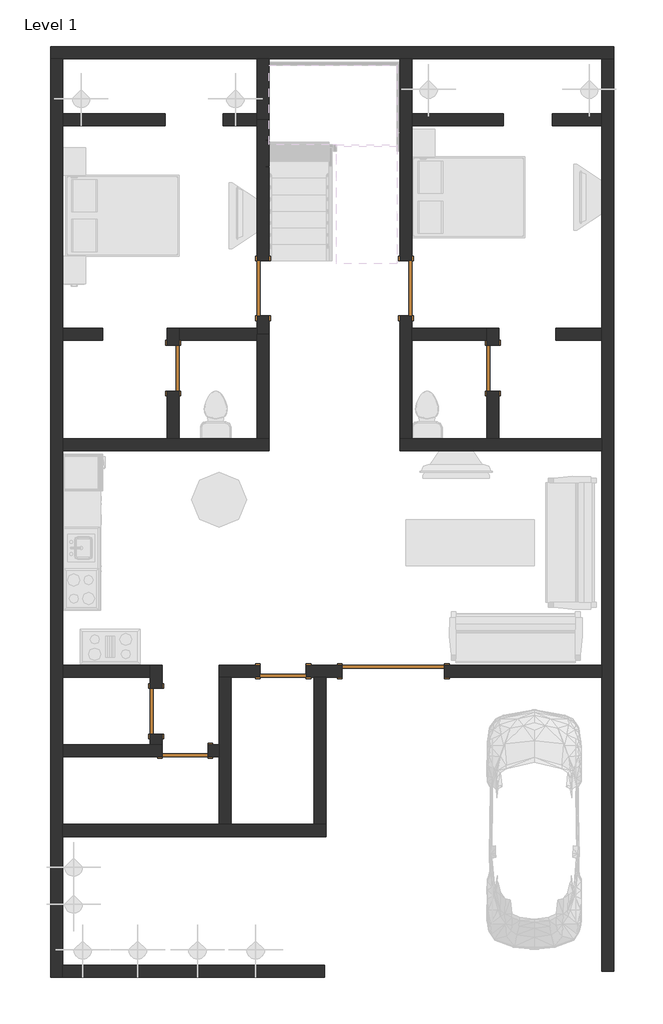
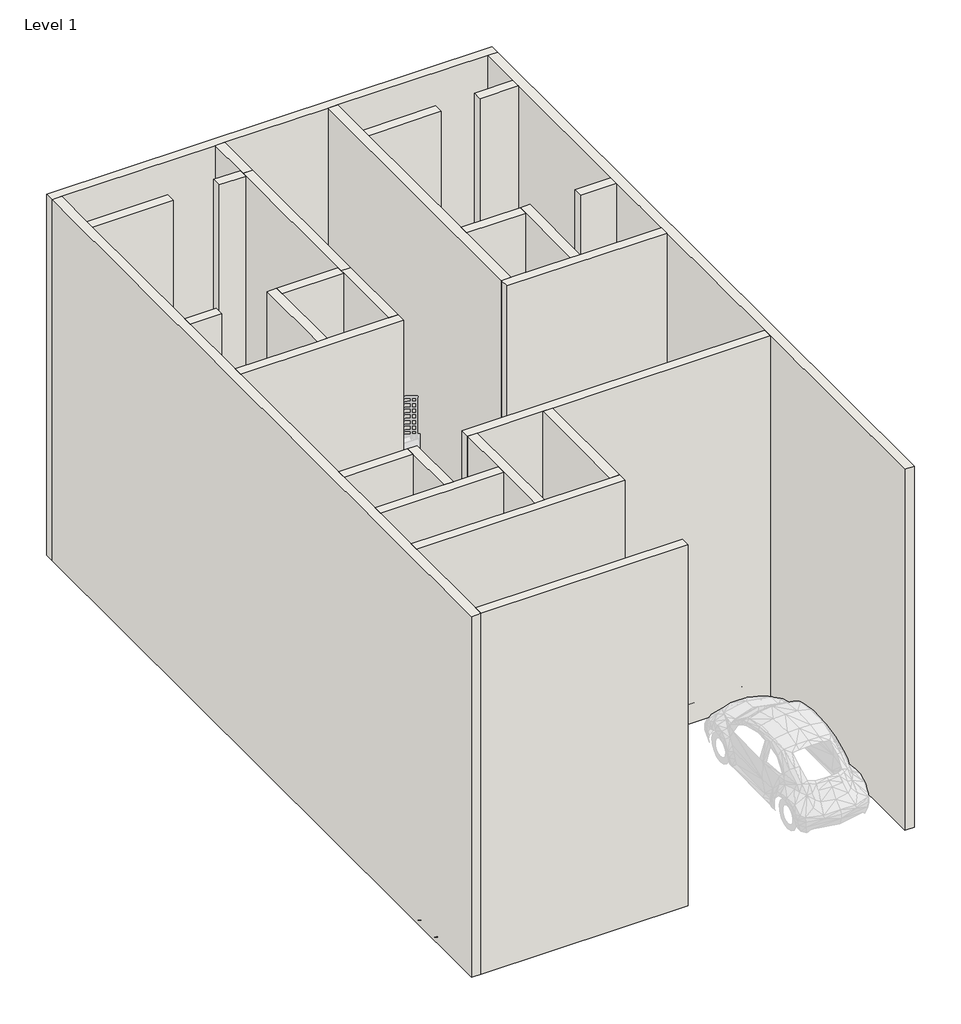
# One storey, part 1 of 4: 27 walls, 8 doors.
"""IFC4 building model written with IfcOpenShell, lengths in millimetres."""

from ifc_helpers import new_model, si_unit, origin, origin_with_axes, place, context, project, spatial, polyline, outline, extrude, faceted_brep, transform, mapped, element, save
from components import m_door_double_flush_panel_double_acting_1700_x_2000mm_0a6d9c7f, m_single_flush_0762_x_2032mm_7341a4fb, m_single_flush_0762_x_2032mm_0c256fab, m_single_flush_0915_x_2134mm_727434cd, m_single_flush_0915_x_2134mm_6a9e8738

model = new_model("IFC4")

# Units and contexts
model_context = context("Model", 3, world=origin())
ifc_project = project(units=[si_unit("LENGTHUNIT", "METRE", prefix="MILLI")], contexts=[model_context])

# Site, building, storey
site = spatial("IfcSite", under=ifc_project)
building = spatial("IfcBuilding", under=site)
storey = spatial("IfcBuildingStorey", under=building, Name="Level 1", Elevation=0.0)

# Doors
placement = place(None, origin())
m_door_double_flush_panel_double_acting_1700_x_2000mm_shape = m_door_double_flush_panel_double_acting_1700_x_2000mm_0a6d9c7f(model_context)
element("IfcDoor", 1, ObjectType="M_Door-Double-Flush_Panel-Double-Acting : 1700 x 2000mm", at=placement, inside=storey, context=model_context, shape_type="MappedRepresentation", body=[
    mapped(m_door_double_flush_panel_double_acting_1700_x_2000mm_shape, transform((-2495.9697318, 2089.9482221, 0.0), x_axis=(1.0, 0.0, 0.0), y_axis=(0.0, 1.0, 0.0), z_axis=(0.0, 0.0, 1.0))),
])
m_single_flush_0762_x_2032mm_shape = m_single_flush_0762_x_2032mm_7341a4fb(model_context)
element("IfcDoor", 2, ObjectType="M_Single-Flush : 0762 x 2032mm", at=placement, inside=storey, context=model_context, shape_type="MappedRepresentation", body=[
    mapped(m_single_flush_0762_x_2032mm_shape, transform((-6155.1697318, 7120.7482221, 0.0), x_axis=(0.0, 1.0, 0.0), y_axis=(-1.0, 0.0, 0.0), z_axis=(0.0, 0.0, 1.0))),
])
element("IfcDoor", 3, ObjectType="M_Single-Flush : 0762 x 2032mm", at=placement, inside=storey, context=model_context, shape_type="MappedRepresentation", body=[
    mapped(m_single_flush_0762_x_2032mm_shape, transform((-5951.9697318, 770.7482221, 0.0), x_axis=(1.0, 0.0, 0.0), y_axis=(0.0, 1.0, 0.0), z_axis=(0.0, 0.0, 1.0))),
])
element("IfcDoor", 4, ObjectType="M_Single-Flush : 0762 x 2032mm", at=placement, inside=storey, context=model_context, shape_type="MappedRepresentation", body=[
    mapped(m_single_flush_0762_x_2032mm_shape, transform((-4324.7697318, 2089.9482221, 0.0), x_axis=(1.0, 0.0, 0.0), y_axis=(0.0, 1.0, 0.0), z_axis=(0.0, 0.0, 1.0))),
])
m_single_flush_0762_x_2032mm_2_shape = m_single_flush_0762_x_2032mm_0c256fab(model_context)
element("IfcDoor", 5, ObjectType="M_Single-Flush : 0762 x 2032mm", at=placement, inside=storey, context=model_context, shape_type="MappedRepresentation", body=[
    mapped(m_single_flush_0762_x_2032mm_2_shape, transform((-844.9697318, 7120.7482221, 0.0), x_axis=(0.0, 1.0, 0.0), y_axis=(-1.0, 0.0, 0.0), z_axis=(0.0, 0.0, 1.0))),
])
element("IfcDoor", 6, ObjectType="M_Single-Flush : 0762 x 2032mm", at=placement, inside=storey, context=model_context, shape_type="MappedRepresentation", body=[
    mapped(m_single_flush_0762_x_2032mm_2_shape, transform((-6434.5697318, 1430.3482221, 0.0), x_axis=(0.0, 1.0, 0.0), y_axis=(-1.0, 0.0, 0.0), z_axis=(0.0, 0.0, 1.0))),
])
m_single_flush_0915_x_2134mm_shape = m_single_flush_0915_x_2134mm_727434cd(model_context)
element("IfcDoor", 7, ObjectType="M_Single-Flush : 0915 x 2134mm", at=placement, inside=storey, context=model_context, shape_type="MappedRepresentation", body=[
    mapped(m_single_flush_0915_x_2134mm_shape, transform((-4662.9197318, 8441.5482221, 0.0), x_axis=(0.0, -1.0, 0.0), y_axis=(1.0, 0.0, 0.0), z_axis=(0.0, 0.0, 1.0))),
])
m_single_flush_0915_x_2134mm_2_shape = m_single_flush_0915_x_2134mm_6a9e8738(model_context)
element("IfcDoor", 8, ObjectType="M_Single-Flush : 0915 x 2134mm", at=placement, inside=storey, context=model_context, shape_type="MappedRepresentation", body=[
    mapped(m_single_flush_0915_x_2134mm_2_shape, transform((-2291.1697318, 8441.5482221, 0.0), x_axis=(0.0, -1.0, 0.0), y_axis=(1.0, 0.0, 0.0), z_axis=(0.0, 0.0, 1.0))),
])

# Walls
element("IfcWall", 9, ObjectType="Generic - 200mm", at=placement, inside=storey, context=model_context, shape_type="Brep", body=[
    faceted_brep([(-8183.9697318, 12253.1482221, 0.0), (-7983.9697318, 12253.1482221, 0.0), (-4761.3197318, 12253.1482221, 0.0), (-4561.3197318, 12253.1482221, 0.0), (-2391.1697318, 12253.1482221, 0.0), (-2191.1697318, 12253.1482221, 0.0), (960.0302682, 12253.1482221, 0.0), (1160.0302682, 12253.1482221, 0.0), (1160.0302682, 12253.1482221, 8000.0), (960.0302682, 12253.1482221, 8000.0), (-2191.1697318, 12253.1482221, 8000.0), (-2391.1697318, 12253.1482221, 8000.0), (-4561.3197318, 12253.1482221, 8000.0), (-4761.3197318, 12253.1482221, 8000.0), (-7983.9697318, 12253.1482221, 8000.0), (-8183.9697318, 12253.1482221, 8000.0), (-8183.9697318, 12453.1482221, 0.0), (-8183.9697318, 12453.1482221, 8000.0), (1160.0302682, 12453.1482221, 8000.0), (1160.0302682, 12453.1482221, 0.0)], [[[0, 1, 2, 3, 4, 5, 6, 7, 8, 9, 10, 11, 12, 13, 14, 15]], [[16, 17, 18, 19]], [[7, 6, 5, 4, 3, 2, 1, 0, 16, 19]], [[15, 14, 13, 12, 11, 10, 9, 8, 18, 17]], [[8, 7, 19, 18]], [[0, 15, 17, 16]]]),
])
element("IfcWall", 10, ObjectType="Generic - 200mm", at=placement, inside=storey, context=model_context, shape_type="Brep", body=[
    faceted_brep([(960.0302682, 12253.1482221, 0.0), (960.0302682, 11335.5482221, 0.0), (960.0302682, 11135.5482221, 0.0), (960.0302682, 7779.5482221, 0.0), (960.0302682, 7579.5482221, 0.0), (960.0302682, 5950.7482221, 0.0), (960.0302682, 5750.7482221, 0.0), (960.0302682, 2189.9482221, 0.0), (960.0302682, 1989.9482221, 0.0), (960.0302682, -2886.8517779, 0.0), (960.0302682, -2886.8517779, 8000.0), (960.0302682, 1989.9482221, 8000.0), (960.0302682, 2189.9482221, 8000.0), (960.0302682, 5750.7482221, 8000.0), (960.0302682, 5950.7482221, 8000.0), (960.0302682, 7579.5482221, 8000.0), (960.0302682, 7779.5482221, 8000.0), (960.0302682, 11135.5482221, 8000.0), (960.0302682, 11335.5482221, 8000.0), (960.0302682, 12253.1482221, 8000.0), (1160.0302682, 12253.1482221, 0.0), (1160.0302682, 12253.1482221, 8000.0), (1160.0302682, -2886.8517779, 8000.0), (1160.0302682, -2886.8517779, 0.0)], [[[0, 1, 2, 3, 4, 5, 6, 7, 8, 9, 10, 11, 12, 13, 14, 15, 16, 17, 18, 19]], [[20, 21, 22, 23]], [[9, 8, 7, 6, 5, 4, 3, 2, 1, 0, 20, 23]], [[10, 9, 23, 22]], [[19, 18, 17, 16, 15, 14, 13, 12, 11, 10, 22, 21]], [[0, 19, 21, 20]]]),
])
element("IfcWall", 11, ObjectType="Generic - 200mm", at=placement, inside=storey, context=model_context, shape_type="Brep", body=[
    faceted_brep([(-7983.9697318, -2986.8517779, 0.0), (-7983.9697318, -2786.8517779, 0.0), (-7983.9697318, -650.0517779, 0.0), (-7983.9697318, -450.0517779, 0.0), (-7983.9697318, 670.7482221, 0.0), (-7983.9697318, 870.7482221, 0.0), (-7983.9697318, 1989.9482221, 0.0), (-7983.9697318, 2189.9482221, 0.0), (-7983.9697318, 5750.7482221, 0.0), (-7983.9697318, 5950.7482221, 0.0), (-7983.9697318, 7579.5482221, 0.0), (-7983.9697318, 7779.5482221, 0.0), (-7983.9697318, 11135.5482221, 0.0), (-7983.9697318, 11335.5482221, 0.0), (-7983.9697318, 12253.1482221, 0.0), (-7983.9697318, 12253.1482221, 8000.0), (-7983.9697318, 11335.5482221, 8000.0), (-7983.9697318, 11135.5482221, 8000.0), (-7983.9697318, 7779.5482221, 8000.0), (-7983.9697318, 7579.5482221, 8000.0), (-7983.9697318, 5950.7482221, 8000.0), (-7983.9697318, 5750.7482221, 8000.0), (-7983.9697318, 2189.9482221, 8000.0), (-7983.9697318, 1989.9482221, 8000.0), (-7983.9697318, 870.7482221, 8000.0), (-7983.9697318, 670.7482221, 8000.0), (-7983.9697318, -450.0517779, 8000.0), (-7983.9697318, -650.0517779, 8000.0), (-7983.9697318, -2786.8517779, 8000.0), (-7983.9697318, -2986.8517779, 8000.0), (-8183.9697318, -2986.8517779, 0.0), (-8183.9697318, -2986.8517779, 8000.0), (-8183.9697318, 12253.1482221, 8000.0), (-8183.9697318, 12253.1482221, 0.0)], [[[0, 1, 2, 3, 4, 5, 6, 7, 8, 9, 10, 11, 12, 13, 14, 15, 16, 17, 18, 19, 20, 21, 22, 23, 24, 25, 26, 27, 28, 29]], [[30, 31, 32, 33]], [[14, 13, 12, 11, 10, 9, 8, 7, 6, 5, 4, 3, 2, 1, 0, 30, 33]], [[29, 28, 27, 26, 25, 24, 23, 22, 21, 20, 19, 18, 17, 16, 15, 32, 31]], [[15, 14, 33, 32]], [[0, 29, 31, 30]]]),
])
element("IfcWall", 12, ObjectType="Generic - 200mm", at=placement, inside=storey, context=model_context, shape_type="Brep", body=[
    faceted_brep([(-4561.3197318, 11235.5482221, 0.0), (-4561.3197318, 12253.1482221, 0.0), (-4561.3197318, 12253.1482221, 8000.0), (-4561.3197318, 11235.5482221, 8000.0), (-4761.3197318, 11235.5482221, 0.0), (-4761.3197318, 11235.5482221, 8000.0), (-4761.3197318, 11335.5482221, 8000.0), (-4761.3197318, 12253.1482221, 8000.0), (-4761.3197318, 12253.1482221, 0.0), (-4761.3197318, 11335.5482221, 0.0), (-4562.9197318, 11235.5482221, 0.0), (-4562.9197318, 11235.5482221, 8000.0)], [[[0, 1, 2, 3]], [[4, 5, 6, 7, 8, 9]], [[1, 0, 10, 4, 9, 8]], [[3, 2, 7, 6, 5, 11]], [[0, 3, 11, 5, 4, 10]], [[2, 1, 8, 7]]]),
])
element("IfcWall", 13, ObjectType="Generic - 200mm", at=placement, inside=storey, context=model_context, shape_type="Brep", body=[
    faceted_brep([(-2191.1697318, 5950.7482221, 0.0), (-2191.1697318, 7579.5482221, 0.0), (-2191.1697318, 7779.5482221, 0.0), (-2191.1697318, 7984.0482221, 0.0), (-2191.1697318, 7984.0482221, 2134.0), (-2191.1697318, 8899.0482221, 2134.0), (-2191.1697318, 8899.0482221, 0.0), (-2191.1697318, 11135.5482221, 0.0), (-2191.1697318, 11335.5482221, 0.0), (-2191.1697318, 12253.1482221, 0.0), (-2191.1697318, 12253.1482221, 8000.0), (-2191.1697318, 11335.5482221, 8000.0), (-2191.1697318, 11135.5482221, 8000.0), (-2191.1697318, 7779.5482221, 8000.0), (-2191.1697318, 7579.5482221, 8000.0), (-2191.1697318, 5950.7482221, 8000.0), (-2391.1697318, 7984.0482221, 2134.0), (-2391.1697318, 7984.0482221, 0.0), (-2391.1697318, 5950.7482221, 0.0), (-2391.1697318, 5950.7482221, 8000.0), (-2391.1697318, 12253.1482221, 8000.0), (-2391.1697318, 12253.1482221, 0.0), (-2391.1697318, 8899.0482221, 0.0), (-2391.1697318, 8899.0482221, 2134.0)], [[[0, 1, 2, 3, 4, 5, 6, 7, 8, 9, 10, 11, 12, 13, 14, 15]], [[16, 17, 18, 19, 20, 21, 22, 23]], [[22, 21, 9, 8, 7, 6]], [[18, 17, 3, 2, 1, 0]], [[15, 14, 13, 12, 11, 10, 20, 19]], [[10, 9, 21, 20]], [[0, 15, 19, 18]], [[4, 3, 17, 16]], [[5, 4, 16, 23]], [[6, 5, 23, 22]]]),
])
element("IfcWall", 14, ObjectType="Generic - 200mm", at=placement, inside=storey, context=model_context, shape_type="Brep", body=[
    faceted_brep([(-4562.9197318, 7679.5482221, 0.0), (-4562.9197318, 7984.0482221, 0.0), (-4562.9197318, 7984.0482221, 2134.0), (-4562.9197318, 8899.0482221, 2134.0), (-4562.9197318, 8899.0482221, 0.0), (-4562.9197318, 11235.5482221, 0.0), (-4562.9197318, 11235.5482221, 8000.0), (-4562.9197318, 7679.5482221, 8000.0), (-4762.9197318, 7984.0482221, 2134.0), (-4762.9197318, 7984.0482221, 0.0), (-4762.9197318, 7779.5482221, 0.0), (-4762.9197318, 7679.5482221, 0.0), (-4762.9197318, 7679.5482221, 8000.0), (-4762.9197318, 7779.5482221, 8000.0), (-4762.9197318, 11135.5482221, 8000.0), (-4762.9197318, 11235.5482221, 8000.0), (-4762.9197318, 11235.5482221, 0.0), (-4762.9197318, 11135.5482221, 0.0), (-4762.9197318, 8899.0482221, 0.0), (-4762.9197318, 8899.0482221, 2134.0), (-4761.3197318, 7679.5482221, 0.0), (-4761.3197318, 11235.5482221, 0.0), (-4761.3197318, 11235.5482221, 8000.0), (-4761.3197318, 7679.5482221, 8000.0)], [[[0, 1, 2, 3, 4, 5, 6, 7]], [[8, 9, 10, 11, 12, 13, 14, 15, 16, 17, 18, 19]], [[11, 10, 9, 1, 0, 20]], [[18, 17, 16, 21, 5, 4]], [[6, 5, 21, 16, 15, 22]], [[7, 6, 22, 15, 14, 13, 12, 23]], [[0, 7, 23, 12, 11, 20]], [[2, 1, 9, 8]], [[3, 2, 8, 19]], [[4, 3, 19, 18]]]),
])
element("IfcWall", 15, ObjectType="Generic - 200mm", at=placement, inside=storey, context=model_context, shape_type="Brep", body=[
    faceted_brep([(-7983.9697318, 5750.7482221, 0.0), (-4561.3197318, 5750.7482221, 0.0), (-4561.3197318, 5750.7482221, 8000.0), (-7983.9697318, 5750.7482221, 8000.0), (-7983.9697318, 5950.7482221, 0.0), (-7983.9697318, 5950.7482221, 8000.0), (-6255.1697318, 5950.7482221, 8000.0), (-6055.1697318, 5950.7482221, 8000.0), (-4761.3197318, 5950.7482221, 8000.0), (-4561.3197318, 5950.7482221, 8000.0), (-4561.3197318, 5950.7482221, 0.0), (-4761.3197318, 5950.7482221, 0.0), (-6055.1697318, 5950.7482221, 0.0), (-6255.1697318, 5950.7482221, 0.0)], [[[0, 1, 2, 3]], [[4, 5, 6, 7, 8, 9, 10, 11, 12, 13]], [[1, 0, 4, 13, 12, 11, 10]], [[3, 2, 9, 8, 7, 6, 5]], [[0, 3, 5, 4]], [[2, 1, 10, 9]]]),
])
element("IfcWall", 16, ObjectType="Generic - 200mm", at=placement, inside=storey, context=model_context, shape_type="Brep", body=[
    faceted_brep([(-6055.1697318, 7501.7482221, 2032.0), (-6055.1697318, 7501.7482221, 0.0), (-6055.1697318, 7579.5482221, 0.0), (-6055.1697318, 7779.5482221, 0.0), (-6055.1697318, 7779.5482221, 8000.0), (-6055.1697318, 7579.5482221, 8000.0), (-6055.1697318, 5950.7482221, 8000.0), (-6055.1697318, 5950.7482221, 0.0), (-6055.1697318, 6739.7482221, 0.0), (-6055.1697318, 6739.7482221, 2032.0), (-6255.1697318, 7779.5482221, 0.0), (-6255.1697318, 7501.7482221, 0.0), (-6255.1697318, 7501.7482221, 2032.0), (-6255.1697318, 6739.7482221, 2032.0), (-6255.1697318, 6739.7482221, 0.0), (-6255.1697318, 5950.7482221, 0.0), (-6255.1697318, 5950.7482221, 8000.0), (-6255.1697318, 7779.5482221, 8000.0)], [[[0, 1, 2, 3, 4, 5, 6, 7, 8, 9]], [[10, 11, 12, 13, 14, 15, 16, 17]], [[8, 7, 15, 14]], [[3, 2, 1, 11, 10]], [[6, 5, 4, 17, 16]], [[7, 6, 16, 15]], [[12, 11, 1, 0]], [[13, 12, 0, 9]], [[14, 13, 9, 8]], [[4, 3, 10, 17]]]),
])
element("IfcWall", 17, ObjectType="Generic - 200mm", at=placement, inside=storey, context=model_context, shape_type="Brep", body=[
    faceted_brep([(-4561.3197318, 5950.7482221, 0.0), (-4561.3197318, 7679.5482221, 0.0), (-4561.3197318, 7679.5482221, 8000.0), (-4561.3197318, 5950.7482221, 8000.0), (-4761.3197318, 5950.7482221, 0.0), (-4761.3197318, 5950.7482221, 8000.0), (-4761.3197318, 7579.5482221, 8000.0), (-4761.3197318, 7679.5482221, 8000.0), (-4761.3197318, 7679.5482221, 0.0), (-4761.3197318, 7579.5482221, 0.0), (-4562.9197318, 7679.5482221, 0.0), (-4562.9197318, 7679.5482221, 8000.0)], [[[0, 1, 2, 3]], [[4, 5, 6, 7, 8, 9]], [[1, 0, 4, 9, 8, 10]], [[2, 1, 10, 8, 7, 11]], [[3, 2, 11, 7, 6, 5]], [[0, 3, 5, 4]]]),
])
element("IfcWall", 18, ObjectType="Generic - 200mm", at=placement, inside=storey, context=model_context, shape_type="Brep", body=[
    faceted_brep([(960.0302682, 5950.7482221, 0.0), (-744.9697318, 5950.7482221, 0.0), (-944.9697318, 5950.7482221, 0.0), (-2191.1697318, 5950.7482221, 0.0), (-2391.1697318, 5950.7482221, 0.0), (-2391.1697318, 5950.7482221, 8000.0), (-2191.1697318, 5950.7482221, 8000.0), (-944.9697318, 5950.7482221, 8000.0), (-744.9697318, 5950.7482221, 8000.0), (960.0302682, 5950.7482221, 8000.0), (960.0302682, 5750.7482221, 0.0), (960.0302682, 5750.7482221, 8000.0), (-2391.1697318, 5750.7482221, 8000.0), (-2391.1697318, 5750.7482221, 0.0)], [[[0, 1, 2, 3, 4, 5, 6, 7, 8, 9]], [[10, 11, 12, 13]], [[4, 3, 2, 1, 0, 10, 13]], [[9, 8, 7, 6, 5, 12, 11]], [[0, 9, 11, 10]], [[5, 4, 13, 12]]]),
])
element("IfcWall", 19, ObjectType="Generic - 200mm", at=placement, inside=storey, context=model_context, shape_type="Brep", body=[
    faceted_brep([(-744.9697318, 7501.7482221, 2032.0), (-744.9697318, 7501.7482221, 0.0), (-744.9697318, 7779.5482221, 0.0), (-744.9697318, 7779.5482221, 8000.0), (-744.9697318, 5950.7482221, 8000.0), (-744.9697318, 5950.7482221, 0.0), (-744.9697318, 6739.7482221, 0.0), (-744.9697318, 6739.7482221, 2032.0), (-944.9697318, 7779.5482221, 0.0), (-944.9697318, 7579.5482221, 0.0), (-944.9697318, 7501.7482221, 0.0), (-944.9697318, 7501.7482221, 2032.0), (-944.9697318, 6739.7482221, 2032.0), (-944.9697318, 6739.7482221, 0.0), (-944.9697318, 5950.7482221, 0.0), (-944.9697318, 5950.7482221, 8000.0), (-944.9697318, 7579.5482221, 8000.0), (-944.9697318, 7779.5482221, 8000.0)], [[[0, 1, 2, 3, 4, 5, 6, 7]], [[8, 9, 10, 11, 12, 13, 14, 15, 16, 17]], [[6, 5, 14, 13]], [[2, 1, 10, 9, 8]], [[4, 3, 17, 16, 15]], [[5, 4, 15, 14]], [[11, 10, 1, 0]], [[12, 11, 0, 7]], [[13, 12, 7, 6]], [[3, 2, 8, 17]]]),
])
element("IfcWall", 20, ObjectType="Generic - 200mm", at=placement, inside=storey, context=model_context, shape_type="Brep", body=[
    faceted_brep([(-7983.9697318, -650.0517779, 0.0), (-3615.1697318, -650.0517779, 0.0), (-3615.1697318, -650.0517779, 8000.0), (-7983.9697318, -650.0517779, 8000.0), (-7983.9697318, -450.0517779, 0.0), (-7983.9697318, -450.0517779, 8000.0), (-5391.5697318, -450.0517779, 8000.0), (-5191.5697318, -450.0517779, 8000.0), (-3815.1697318, -450.0517779, 8000.0), (-3615.1697318, -450.0517779, 8000.0), (-3615.1697318, -450.0517779, 0.0), (-3815.1697318, -450.0517779, 0.0), (-5191.5697318, -450.0517779, 0.0), (-5391.5697318, -450.0517779, 0.0)], [[[0, 1, 2, 3]], [[4, 5, 6, 7, 8, 9, 10, 11, 12, 13]], [[1, 0, 4, 13, 12, 11, 10]], [[3, 2, 9, 8, 7, 6, 5]], [[0, 3, 5, 4]], [[2, 1, 10, 9]]]),
])
element("IfcWall", 21, ObjectType="Generic - 200mm", at=placement, inside=storey, context=model_context, shape_type="Brep", body=[
    faceted_brep([(-5570.9697318, 670.7482221, 2032.0), (-5570.9697318, 670.7482221, 0.0), (-5391.5697318, 670.7482221, 0.0), (-5391.5697318, 670.7482221, 8000.0), (-7983.9697318, 670.7482221, 8000.0), (-7983.9697318, 670.7482221, 0.0), (-6332.9697318, 670.7482221, 0.0), (-6332.9697318, 670.7482221, 2032.0), (-5391.5697318, 870.7482221, 0.0), (-5570.9697318, 870.7482221, 0.0), (-5570.9697318, 870.7482221, 2032.0), (-6332.9697318, 870.7482221, 2032.0), (-6332.9697318, 870.7482221, 0.0), (-6334.5697318, 870.7482221, 0.0), (-6534.5697318, 870.7482221, 0.0), (-7983.9697318, 870.7482221, 0.0), (-7983.9697318, 870.7482221, 8000.0), (-6534.5697318, 870.7482221, 8000.0), (-6334.5697318, 870.7482221, 8000.0), (-5391.5697318, 870.7482221, 8000.0)], [[[0, 1, 2, 3, 4, 5, 6, 7]], [[8, 9, 10, 11, 12, 13, 14, 15, 16, 17, 18, 19]], [[6, 5, 15, 14, 13, 12]], [[2, 1, 9, 8]], [[4, 3, 19, 18, 17, 16]], [[5, 4, 16, 15]], [[3, 2, 8, 19]], [[10, 9, 1, 0]], [[11, 10, 0, 7]], [[12, 11, 7, 6]]]),
])
element("IfcWall", 22, ObjectType="Generic - 200mm", at=placement, inside=storey, context=model_context, shape_type="Brep", body=[
    faceted_brep([(-5391.5697318, 1989.9482221, 0.0), (-5391.5697318, 870.7482221, 0.0), (-5391.5697318, 670.7482221, 0.0), (-5391.5697318, -450.0517779, 0.0), (-5391.5697318, -450.0517779, 8000.0), (-5391.5697318, 670.7482221, 8000.0), (-5391.5697318, 870.7482221, 8000.0), (-5391.5697318, 1989.9482221, 8000.0), (-5191.5697318, 1989.9482221, 0.0), (-5191.5697318, 1989.9482221, 8000.0), (-5191.5697318, -450.0517779, 8000.0), (-5191.5697318, -450.0517779, 0.0)], [[[0, 1, 2, 3, 4, 5, 6, 7]], [[8, 9, 10, 11]], [[3, 2, 1, 0, 8, 11]], [[7, 6, 5, 4, 10, 9]], [[4, 3, 11, 10]], [[0, 7, 9, 8]]]),
])
element("IfcWall", 23, ObjectType="Generic - 200mm", at=placement, inside=storey, context=model_context, shape_type="Brep", body=[
    faceted_brep([(-6334.5697318, 1811.3482221, 2032.0), (-6334.5697318, 1811.3482221, 0.0), (-6334.5697318, 2189.9482221, 0.0), (-6334.5697318, 2189.9482221, 8000.0), (-6334.5697318, 870.7482221, 8000.0), (-6334.5697318, 870.7482221, 0.0), (-6334.5697318, 1049.3482221, 0.0), (-6334.5697318, 1049.3482221, 2032.0), (-6534.5697318, 2189.9482221, 0.0), (-6534.5697318, 1989.9482221, 0.0), (-6534.5697318, 1811.3482221, 0.0), (-6534.5697318, 1811.3482221, 2032.0), (-6534.5697318, 1049.3482221, 2032.0), (-6534.5697318, 1049.3482221, 0.0), (-6534.5697318, 870.7482221, 0.0), (-6534.5697318, 870.7482221, 8000.0), (-6534.5697318, 1989.9482221, 8000.0), (-6534.5697318, 2189.9482221, 8000.0)], [[[0, 1, 2, 3, 4, 5, 6, 7]], [[8, 9, 10, 11, 12, 13, 14, 15, 16, 17]], [[6, 5, 14, 13]], [[2, 1, 10, 9, 8]], [[4, 3, 17, 16, 15]], [[5, 4, 15, 14]], [[3, 2, 8, 17]], [[11, 10, 1, 0]], [[12, 11, 0, 7]], [[13, 12, 7, 6]]]),
])
element("IfcWall", 24, ObjectType="Generic - 200mm", at=placement, inside=storey, context=model_context, shape_type="SweptSolid", body=[
    extrude(outline(polyline([(-7983.9697318, 2189.9482221), (-6534.5697318, 2189.9482221), (-6534.5697318, 1989.9482221), (-7983.9697318, 1989.9482221), (-7983.9697318, 2189.9482221)])), origin_with_axes(), (0.0, 0.0, 1.0), 8000.0),
])
element("IfcWall", 25, ObjectType="Generic - 200mm", at=placement, inside=storey, context=model_context, shape_type="Brep", body=[
    faceted_brep([(-5391.5697318, 2189.9482221, 8000.0), (960.0302682, 2189.9482221, 8000.0), (960.0302682, 2189.9482221, 0.0), (-1645.9697318, 2189.9482221, 0.0), (-1645.9697318, 2189.9482221, 2000.0), (-3345.9697318, 2189.9482221, 2000.0), (-3345.9697318, 2189.9482221, 0.0), (-3943.7697318, 2189.9482221, 0.0), (-3943.7697318, 2189.9482221, 2032.0), (-4705.7697318, 2189.9482221, 2032.0), (-4705.7697318, 2189.9482221, 0.0), (-5391.5697318, 2189.9482221, 0.0), (960.0302682, 1989.9482221, 8000.0), (-3615.1697318, 1989.9482221, 8000.0), (-3815.1697318, 1989.9482221, 8000.0), (-5191.5697318, 1989.9482221, 8000.0), (-5391.5697318, 1989.9482221, 8000.0), (-5391.5697318, 1989.9482221, 0.0), (-5191.5697318, 1989.9482221, 0.0), (-4705.7697318, 1989.9482221, 0.0), (-4705.7697318, 1989.9482221, 2032.0), (-3943.7697318, 1989.9482221, 2032.0), (-3943.7697318, 1989.9482221, 0.0), (-3815.1697318, 1989.9482221, 0.0), (-3615.1697318, 1989.9482221, 0.0), (-3345.9697318, 1989.9482221, 0.0), (-3345.9697318, 1989.9482221, 2000.0), (-1645.9697318, 1989.9482221, 2000.0), (-1645.9697318, 1989.9482221, 0.0), (960.0302682, 1989.9482221, 0.0)], [[[0, 1, 2, 3, 4, 5, 6, 7, 8, 9, 10, 11]], [[12, 13, 14, 15, 16, 17, 18, 19, 20, 21, 22, 23, 24, 25, 26, 27, 28, 29]], [[17, 11, 10, 19, 18]], [[2, 29, 28, 3]], [[22, 7, 6, 25, 24, 23]], [[1, 0, 16, 15, 14, 13, 12]], [[0, 11, 17, 16]], [[2, 1, 12, 29]], [[8, 7, 22, 21]], [[9, 8, 21, 20]], [[10, 9, 20, 19]], [[27, 4, 3, 28]], [[4, 27, 26, 5]], [[5, 26, 25, 6]]]),
])
element("IfcWall", 26, ObjectType="Generic - 200mm", at=placement, inside=storey, context=model_context, shape_type="SweptSolid", body=[
    extrude(outline(polyline([(-3815.1697318, -450.0517779), (-3815.1697318, 1989.9482221), (-3615.1697318, 1989.9482221), (-3615.1697318, -450.0517779), (-3815.1697318, -450.0517779)])), origin_with_axes(), (0.0, 0.0, 1.0), 8000.0),
])
element("IfcWall", 27, ObjectType="Generic - 200mm", at=placement, inside=storey, context=model_context, shape_type="SweptSolid", body=[
    extrude(outline(polyline([(-6055.1697318, 7779.5482221), (-4762.9197318, 7779.5482221), (-4762.9197318, 7679.5482221), (-4761.3197318, 7679.5482221), (-4761.3197318, 7579.5482221), (-6055.1697318, 7579.5482221), (-6055.1697318, 7779.5482221)])), origin_with_axes(), (0.0, 0.0, 1.0), 8000.0),
])
element("IfcWall", 28, ObjectType="Generic - 200mm", at=placement, inside=storey, context=model_context, shape_type="SweptSolid", body=[
    extrude(outline(polyline([(-7323.5697318, 7579.5482221), (-7983.9697318, 7579.5482221), (-7983.9697318, 7779.5482221), (-7323.5697318, 7779.5482221), (-7323.5697318, 7579.5482221)])), origin_with_axes(), (0.0, 0.0, 1.0), 8000.0),
])
element("IfcWall", 29, ObjectType="Generic - 200mm", at=placement, inside=storey, context=model_context, shape_type="SweptSolid", body=[
    extrude(outline(polyline([(-944.9697318, 7579.5482221), (-2191.1697318, 7579.5482221), (-2191.1697318, 7779.5482221), (-944.9697318, 7779.5482221), (-944.9697318, 7579.5482221)])), origin_with_axes(), (0.0, 0.0, 1.0), 8000.0),
])
element("IfcWall", 30, ObjectType="Generic - 200mm", at=placement, inside=storey, context=model_context, shape_type="SweptSolid", body=[
    extrude(outline(polyline([(198.0302682, 7779.5482221), (960.0302682, 7779.5482221), (960.0302682, 7579.5482221), (198.0302682, 7579.5482221), (198.0302682, 7779.5482221)])), origin_with_axes(), (0.0, 0.0, 1.0), 8000.0),
])
element("IfcWall", 31, ObjectType="Generic - 200mm", at=placement, inside=storey, context=model_context, shape_type="SweptSolid", body=[
    extrude(outline(polyline([(-6283.7697318, 11135.5482221), (-7983.9697318, 11135.5482221), (-7983.9697318, 11335.5482221), (-6283.7697318, 11335.5482221), (-6283.7697318, 11135.5482221)])), origin_with_axes(), (0.0, 0.0, 1.0), 8000.0),
])
element("IfcWall", 32, ObjectType="Generic - 200mm", at=placement, inside=storey, context=model_context, shape_type="SweptSolid", body=[
    extrude(outline(polyline([(-667.1697318, 11135.5482221), (-2191.1697318, 11135.5482221), (-2191.1697318, 11335.5482221), (-667.1697318, 11335.5482221), (-667.1697318, 11135.5482221)])), origin_with_axes(), (0.0, 0.0, 1.0), 8000.0),
])
element("IfcWall", 33, ObjectType="Generic - 200mm", at=placement, inside=storey, context=model_context, shape_type="SweptSolid", body=[
    extrude(outline(polyline([(960.0302682, 11135.5482221), (145.6302682, 11135.5482221), (145.6302682, 11335.5482221), (960.0302682, 11335.5482221), (960.0302682, 11135.5482221)])), origin_with_axes(), (0.0, 0.0, 1.0), 8000.0),
])
element("IfcWall", 34, ObjectType="Generic - 200mm", at=placement, inside=storey, context=model_context, shape_type="SweptSolid", body=[
    extrude(outline(polyline([(-5321.7197318, 11335.5482221), (-4761.3197318, 11335.5482221), (-4761.3197318, 11235.5482221), (-4762.9197318, 11235.5482221), (-4762.9197318, 11135.5482221), (-5321.7197318, 11135.5482221), (-5321.7197318, 11335.5482221)])), origin_with_axes(), (0.0, 0.0, 1.0), 8000.0),
])
element("IfcWall", 35, ObjectType="Generic - 200mm", at=placement, inside=storey, context=model_context, shape_type="SweptSolid", body=[
    extrude(outline(polyline([(-3640.5697318, -2986.8517779), (-7983.9697318, -2986.8517779), (-7983.9697318, -2786.8517779), (-3640.5697318, -2786.8517779), (-3640.5697318, -2986.8517779)])), origin_with_axes(), (0.0, 0.0, 1.0), 8000.0),
])

save(model, "model.ifc")

# Revit data of these elements
# Type "M_Door-Double-Flush_Panel-Double-Acting : 1700 x 2000mm"
#   Type Mark = "22"
#   Construction Type Id = "DOOR"
#   Assembly Code = "C1020"
#   Analytic Construction = "Wooden"
#   W = 850 mm
#   Thickness = 50 mm
#   Thermal Resistance (R) = 0.455703 (m²·K)/W
#   Swing Angle [instance default] = 90.00°
#   Heat Transfer Coefficient (U) = 2.19465 W/(m²·K)
#   Height = 2000 mm
#   Trim Projection Ext. = 25 mm
#   Trim Projection Int. = 25 mm
#   Trim Width Ext. = 80 mm
#   Trim Width Int. = 80 mm
#   Width = 1700 mm
#   Define Thermal Properties by = 1
#   Panel Material = Wood - Birch - Solid Stained Light Low Gloss
#   Trim Material = Paint - Sienna
#   Visual Light Transmittance = 0
#   Solar Heat Gain Coefficient = 0
#   Function = (empty or 0)
#   Wall Closure = (empty or 0)
# Type "M_Single-Flush : 0762 x 2032mm"
#   Type Mark = "19"
#   Thickness = 51 mm
#   Height = 2032 mm
#   Trim Projection Ext = 25 mm
#   Trim Projection Int = 25 mm
#   Trim Width = 76 mm
#   Width = 762 mm
#   Door Material = Door - Panel
#   Frame Material = Door - Frame
#   Function = (empty or 0)
#   Wall Closure = (empty or 0)
# Type "M_Single-Flush : 0915 x 2134mm"
#   Type Mark = "15"
#   Thickness = 51 mm
#   Height = 2134 mm
#   Trim Projection Ext = 25 mm
#   Trim Projection Int = 25 mm
#   Trim Width = 76 mm
#   Width = 915 mm
#   Door Material = Door - Panel
#   Frame Material = Door - Frame
#   Function = (empty or 0)
#   Wall Closure = (empty or 0)
# Type "Generic - 200mm"
#   Layers, outside or top first: 200 mm no material (function 1)
# Element 1 (IfcDoor, "M_Door-Double-Flush_Panel-Double-Acting : 1700 x 2000mm")
#   Swing Angle = 90.00°
#   Phase Created = New Construction
#   Materials on its faces: "Paint - Sienna", "Wood - Birch - Solid Stained Light Low Gloss"
# Elements 2, 3, 4, 5, 6 (IfcDoor, "M_Single-Flush : 0762 x 2032mm")
#   Phase Created = New Construction
#   Materials on its faces: "Door - Frame", "Door - Panel"
# Elements 7, 8 (IfcDoor, "M_Single-Flush : 0915 x 2134mm")
#   Phase Created = New Construction
#   Materials on its faces: "Door - Frame", "Door - Panel"
# Elements 9, 10, 11, 12, 13, 14, 15, 16, 17, 18, 19, 20, 21, 22, 23, 24, 25, 26, 27, 28, 29, 30, 31, 32, 33, 34, 35 (IfcWall, "Generic - 200mm")
#   Top Offset = 0 mm
#   Base Offset = 0 mm
#   Unconnected Height = 8000 mm
#   wall height = 8000 mm
#   Phase Created = New Construction
#   Base Constraint = Level 1
#   Materials on its faces: "Default Wall"
# Materials
#   "Wood - Birch - Solid Stained Light Low Gloss": class "Wood", colour RGB 210 159 95, transparency 0, Cost = 0
#   "Paint - Sienna": colour RGB 118 70 51, transparency 0, Cost = 0
#   "Door - Panel": class "Wood", colour RGB 114 82 51, transparency 0
#   "Door - Frame": colour RGB 153 76 43, transparency 0
#   "Default Wall": colour RGB 80 80 80, transparency 0
